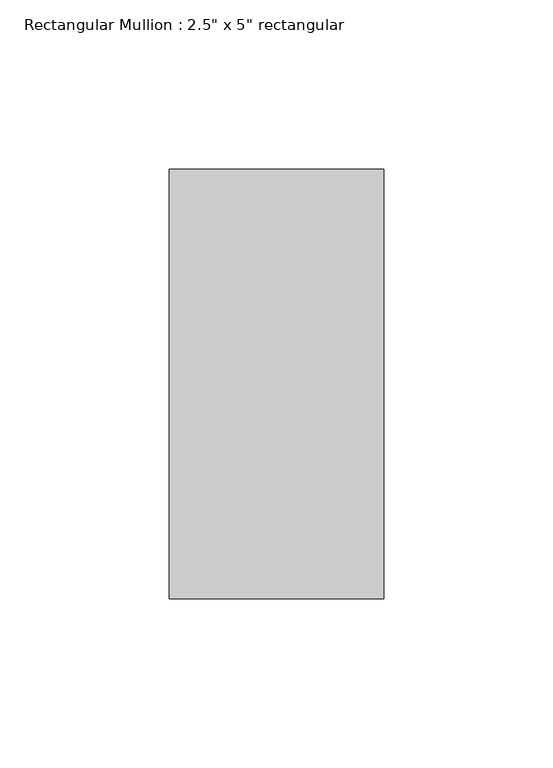
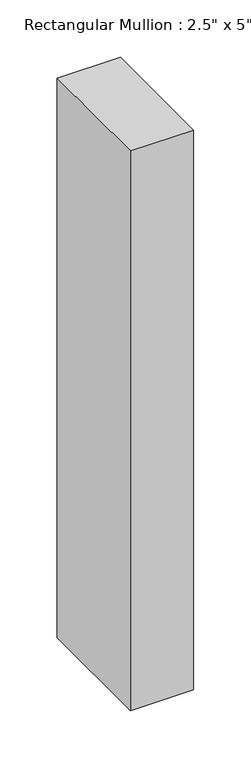
"""IFC4 building model written with IfcOpenShell, lengths in millimetres: member geometry."""

from ifc_helpers import new_model, si_unit, frame, origin, place, context, project, spatial, polyline, outline, extrude, source, transform, mapped, element, save


def member_e44847c7(model_context):
    return source(origin(), model_context, "Body", "SweptSolid", [
        extrude(outline(polyline([(0.0, 63.5), (0.0, -63.5), (-63.5, -63.5), (-63.5, 63.5), (0.0, 63.5)])), frame((0.0, 0.0, -594.0122725), z_axis=(0.0, 0.0, 1.0), x_axis=(1.0, 0.0, 0.0)), (0.0, 0.0, 1.0), 594.0122725),
    ])


if __name__ == "__main__":
    model = new_model("IFC4")
    model_context = context("Model", 3, world=origin())
    ifc_project = project(units=[si_unit("LENGTHUNIT", "METRE", prefix="MILLI")], contexts=[model_context])
    site = spatial("IfcSite", under=ifc_project)
    building = spatial("IfcBuilding", under=site)
    placement = place(None, origin())
    member_shape = member_e44847c7(model_context)
    element("IfcMember", 1, ObjectType="Rectangular Mullion : 2.5\" x 5\" rectangular", at=placement, inside=building, context=model_context, shape_type="MappedRepresentation", body=[
        mapped(member_shape, transform((0.0, 0.0, 0.0), x_axis=(1.0, 0.0, 0.0), y_axis=(0.0, 1.0, 0.0), z_axis=(0.0, 0.0, 1.0))),
    ])
    save(model, "model.ifc")

# Revit data of these elements
# Type "Rectangular Mullion : 2.5\" x 5\" rectangular"
#   built-in parameter 1007304 = 0.416667 (stored number, unit not read)
#   built-in parameter 1007301 = 0.104167 (stored number, unit not read)
#   built-in parameter 1007300 = 0.104167 (stored number, unit not read)
# Element 1 (IfcMember, "Rectangular Mullion : 2.5\" x 5\" rectangular")
#   Materials on its faces: "Aluminum"
# Materials
#   "Aluminum": class "Metal", colour RGB 247 247 247, transparency 0, Description = "Aluminum 6061", Cost = 0
